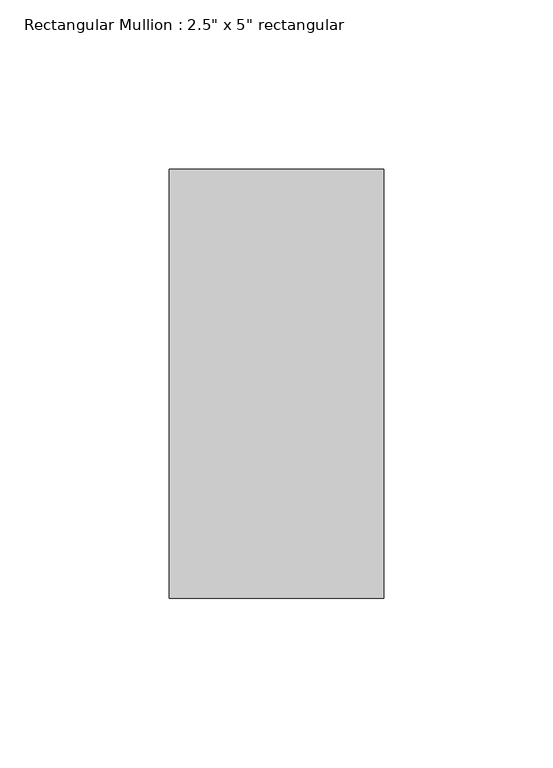
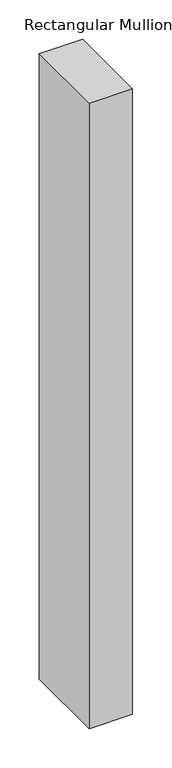
"""IFC4 building model written with IfcOpenShell, lengths in millimetres: member geometry."""

from ifc_helpers import new_model, si_unit, frame, origin, place, context, project, spatial, polyline, outline, extrude, source, transform, mapped, element, save


def member_801a2072(model_context):
    return source(origin(), model_context, "Body", "SweptSolid", [
        extrude(outline(polyline([(0.0, 63.5), (0.0, -63.5), (-63.5, -63.5), (-63.5, 63.5), (0.0, 63.5)])), frame((0.0, 0.0, -971.55), z_axis=(0.0, 0.0, 1.0), x_axis=(1.0, 0.0, 0.0)), (0.0, 0.0, 1.0), 971.55),
    ])


if __name__ == "__main__":
    model = new_model("IFC4")
    model_context = context("Model", 3, world=origin())
    ifc_project = project(units=[si_unit("LENGTHUNIT", "METRE", prefix="MILLI")], contexts=[model_context])
    site = spatial("IfcSite", under=ifc_project)
    building = spatial("IfcBuilding", under=site)
    placement = place(None, origin())
    member_shape = member_801a2072(model_context)
    element("IfcMember", 1, ObjectType="Rectangular Mullion : 2.5\" x 5\" rectangular", at=placement, inside=building, context=model_context, shape_type="MappedRepresentation", body=[
        mapped(member_shape, transform((0.0, 0.0, 0.0), x_axis=(1.0, 0.0, 0.0), y_axis=(0.0, 1.0, 0.0), z_axis=(0.0, 0.0, 1.0))),
    ])
    save(model, "model.ifc")

# Revit data of these elements
# Type "Rectangular Mullion : 2.5\" x 5\" rectangular"
#   built-in parameter 1007304 = 0.416667 (stored number, unit not read)
#   built-in parameter 1007301 = 0.104167 (stored number, unit not read)
#   built-in parameter 1007300 = 0.104167 (stored number, unit not read)
# Element 1 (IfcMember, "Rectangular Mullion : 2.5\" x 5\" rectangular")
#   Materials on its faces: "Iron, Ductile"
# Materials
#   "Iron, Ductile": class "Metal", colour RGB 0 0 0, transparency 0, Description = "Ductile cast iron", Cost = 0
